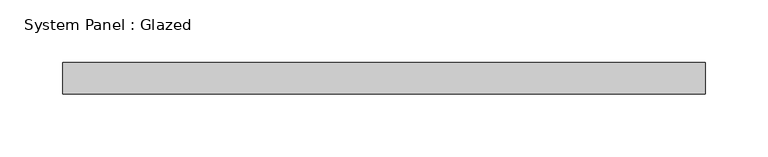
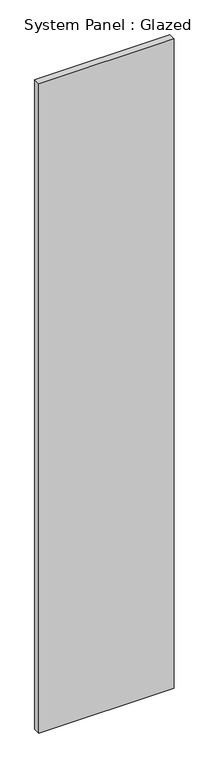
"""IFC4 building model written with IfcOpenShell, lengths in millimetres: plate geometry, System Panel : Glazed."""

from ifc_helpers import new_model, si_unit, origin, origin_with_axes, place, context, project, spatial, polyline, outline, extrude, source, transform, mapped, element, save


def system_panel_glazed_3ff1fc73(model_context):
    return source(origin(), model_context, "Body", "SweptSolid", [
        extrude(outline(polyline([(257.175, 19.05), (-257.175, 19.05), (-257.175, 44.45), (257.175, 44.45), (257.175, 19.05)])), origin_with_axes(), (0.0, 0.0, 1.0), 2609.6448327),
    ])


if __name__ == "__main__":
    model = new_model("IFC4")
    model_context = context("Model", 3, world=origin())
    ifc_project = project(units=[si_unit("LENGTHUNIT", "METRE", prefix="MILLI")], contexts=[model_context])
    site = spatial("IfcSite", under=ifc_project)
    building = spatial("IfcBuilding", under=site)
    placement = place(None, origin())
    system_panel_glazed_shape = system_panel_glazed_3ff1fc73(model_context)
    element("IfcPlate", 1, ObjectType="System Panel : Glazed", at=placement, inside=building, context=model_context, shape_type="MappedRepresentation", body=[
        mapped(system_panel_glazed_shape, transform((0.0, 0.0, 0.0), x_axis=(1.0, 0.0, 0.0), y_axis=(0.0, 1.0, 0.0), z_axis=(0.0, 0.0, 1.0))),
    ])
    save(model, "model.ifc")

# Revit data of these elements
# Type "System Panel : Glazed"
#   Construction Type Id = "GSP4R"
#   Analytic Construction = "1/8 in Pilkington single glazing"
#   Visual Light Transmittance = 0.9
#   Solar Heat Gain Coefficient = 0.86
#   Heat Transfer Coefficient (U) = 1.18115 BTU/(h·ft²·°F)
#   Define Thermal Properties by = 1
# Element 1 (IfcPlate, "System Panel : Glazed")
#   Materials on its faces: "Glass"
# Materials
#   "Glass": class "Glass", colour RGB 0 128 192, transparency 0.75, Description = "Soda Lime Glass", Cost = 0
